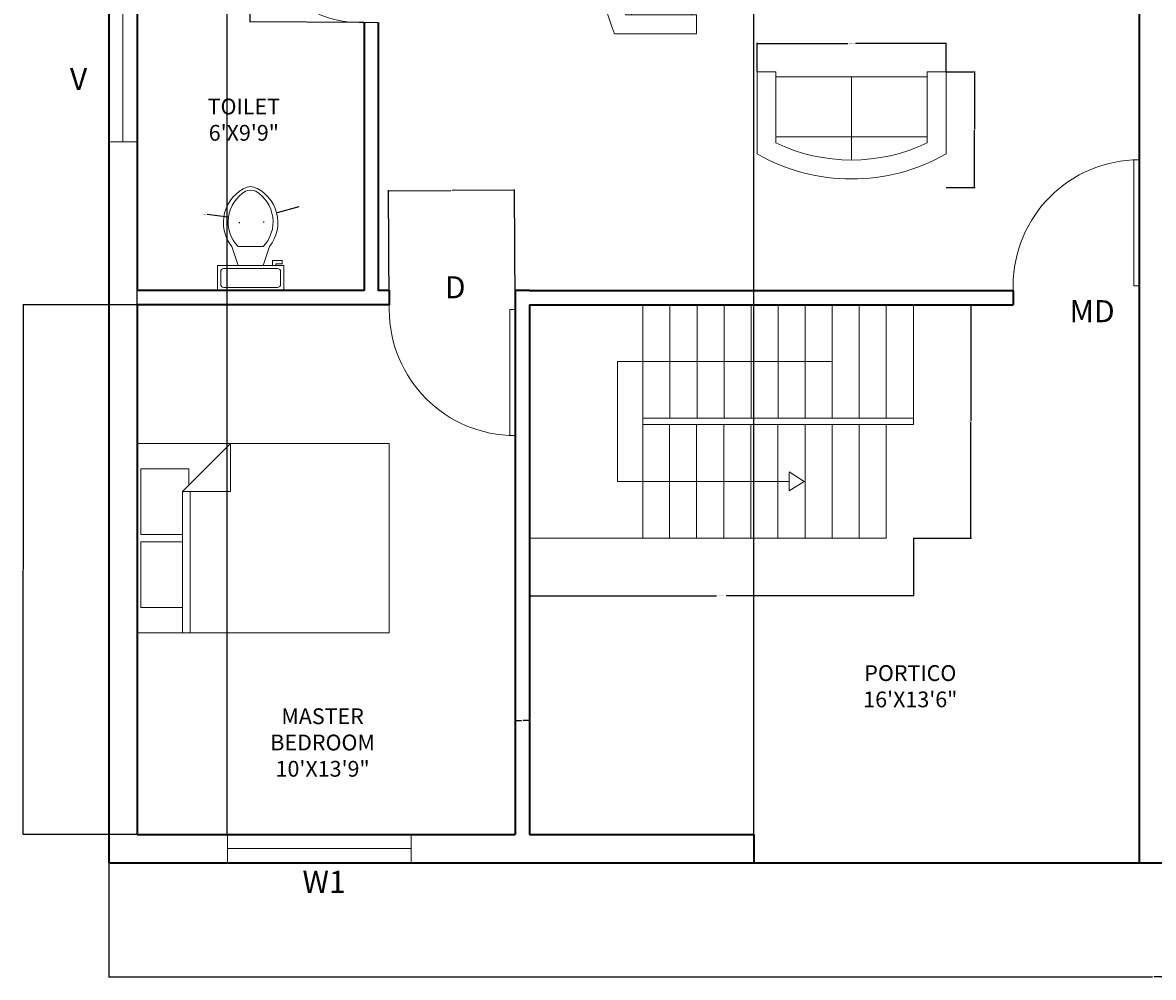
# Model space of a CAD drawing. Units: inches. Extents: x 1939 to 2674, y 558 to 1170.
# Tile 1 of 6: x 1948 to 2307, y 558 to 861. Entities that reach past the tile are written whole.
import ezdxf

# ---------------------------------------------------------------- set-up
doc = ezdxf.new("R2010")
doc.units = ezdxf.units.IN
for name, color, linetype, lineweight in [('A-ANNO-DIMS', 2, 'Continuous', 18), ('A-ANNO-TEXT', 7, 'Continuous', 18), ('A-AREA-IDEN', 7, 'Continuous', 18), ('A-DOOR', 3, 'Continuous', 18), ('A-FLOR-FIXT', 9, 'Continuous', 18), ('A-FLOR-STRS', 7, 'Continuous', 18), ('A-FURN', 8, 'Continuous', 13), ('A-GLAZ', 4, 'Continuous', 18), ('A-WALL', 7, 'Continuous', 35)]:
    doc.layers.add(name, color=color, linetype=linetype, lineweight=lineweight)
doc.styles.get("Standard").update_dxf_attribs({"font": 'arial.ttf'})
doc.dimstyles.get("Standard").update_dxf_attribs({"dimtxt": 0.18, "dimasz": 0.18, "dimexe": 0.18, "dimexo": 0.0625, "dimgap": 0.09, "dimtad": 0, "dimtih": 1, "dimtoh": 1, "dimdec": 4, "dimzin": 0, "dimdsep": 46, "dimtxsty": 'Standard', "dimcen": 0.09, "dimadec": 0, "dimazin": 0, "dimtfac": 1, "dimtdec": 4, "dimtofl": 0, "dimtmove": 0, "dimatfit": 3, "dimfxl": 1, "dimtolj": 1, "dimtzin": 0, "dimarcsym": 0})

# ---------------------------------------------------------------- blocks, each defined once
blk = doc.blocks.new('Sofa - Roundback 7 ft.')
for p, q in [((-12.00002, -32.4421), (-12.00003, -6.5971)), ((11.99997, -32.4421), (11.99998, -6.5971)), ((-36.000027, -34), (-36.000027, -11.4696)), ((-35.999844, -13.3819), (35.9998, -13.3819)), ((35.99998, -34), (35.99998, -11.4696)), ((-36.000027, -32.4421), (35.99998, -32.4421))]:
    blk.add_line(p, q)
for points in [[(-36.000027, -34), (-42.000027, -34), (-42.000027, -8)], [(41.99998, -8), (41.99998, -34), (35.99998, -34)]]:
    blk.add_lwpolyline(points)
for centre, radius, start, end in [((0, -114.25), 114.25, 68.43141, 111.5686), ((-0.00001, -127.1968), 121.1968, 72.72033, 107.2797)]:
    blk.add_arc(centre, radius, start, end)
blk = doc.blocks.new('Toilet - top')
for p, q in [((9.5, -6), (9.5, -2)), ((-10, -8.5), (-8, -8.5)), ((-10, -9.5), (-10, -8.5)), ((-7, -9.5), (-10, -9.5)), ((-8, -8.5), (-8, -8)), ((-7, -8), (-7, -9.5)), ((-4, -8), (-6, -14)), ((4, -8), (6, -14)), ((4, -14), (-4, -14))]:
    blk.add_line(p, q)
blk.add_lwpolyline([(10.5, -8), (10.5, 0), (-10.5, 0), (-10.5, -8)], close=True)
for points in [[(-9.5, -2), (-9.5, -6)], [(8.5, -1), (-8.5, -1)], [(-8.5, -7), (8.5, -7)]]:
    blk.add_lwpolyline(points)
for centre, radius, start, end in [((-8.62, -1.88), 0.884, 81.8699, 188.1301), ((8.62, -1.88), 0.884, 351.8699, 98.1301), ((-8.62, -6.12), 0.884, 171.8699, 278.1301), ((8.62, -6.12), 0.884, 261.8699, 8.1301), ((3.52, -21.58), 12.17, 141.4691, 247.9714), ((4.2, -21.82), 11.33, 136.3677, 238.9468), ((-3.52, -21.58), 12.17, 292.0284, 38.5307), ((-4.2, -21.82), 11.33, 301.053, 43.6321), ((0, -27.88), 4, 245.7318, 294.2682), ((0, -29), 4, 254.8605, 285.1395)]:
    blk.add_arc(centre, radius, start, end)
blk = doc.blocks.new('Bed - Queen')
for p, q in [((0, -80.00003), (0, 0)), ((0, 0), (59.99999, 0)), ((59.99999, 0), (59.99999, -80.00003)), ((7.99999, -1.2), (28.79998, -1.2)), ((7.99999, -14.4), (7.99999, -1.2)), ((28.79998, -1.2), (28.79998, -14.4)), ((31.19999, -1.2), (51.99999, -1.2)), ((31.19999, -14.4), (31.19999, -1.2)), ((51.99999, -1.2), (51.99999, -16.4)), ((0, -14.4), (44.8, -14.4)), ((44.8, -16.8), (0, -16.8)), ((59.99999, -29.6), (44.8, -14.4)), ((44.8, -14.4), (44.8, -29.6)), ((51.99999, -16.4), (46.79936, -16.4)), ((44.8, -29.6), (59.99999, -29.6)), ((59.99999, -80.00003), (0, -80.00003))]:
    blk.add_line(p, q)
blk = doc.blocks.new('Sofa - Roundback Loveseat 5 ft.')
for p, q in [((0, -32.44198), (0, -5.99998)), ((-24, -33.99998), (-24, -11.46958)), ((-23.9998, -13.38178), (23.99986, -13.38178)), ((24.00004, -33.99998), (24.00004, -11.46958)), ((-24, -32.44198), (24.00004, -32.44198))]:
    blk.add_line(p, q)
for points in [[(-24, -33.99998), (-30, -33.99998), (-30, -7.99998)], [(30.00004, -7.99998), (30.00004, -33.99998), (24.00004, -33.99998)]]:
    blk.add_lwpolyline(points)
for centre, radius, start, end in [((0, -60.24998), 60.24998, 60.13715, 119.8628), ((0, -61.38438), 55.38444, 64.32083, 115.6792)]:
    blk.add_arc(centre, radius, start, end)
blk = doc.blocks.new('*U12')
for p, q in [((0, 0), (0, -6)), ((-32, 0), (-32, -6))]:
    blk.add_line(p, q)
blk.add_lwpolyline([(0, 0), (0, 32), (-1.75, 32), (-1.75, 0)], close=True)
blk.add_arc((0, 0), 32, 90, 180)
blk = doc.blocks.new('*U11')
for p, q in [((0, 0), (0, -6)), ((-40, 0), (-40, -6))]:
    blk.add_line(p, q)
blk.add_lwpolyline([(0, 0), (0, 40), (-1.75, 40), (-1.75, 0)], close=True)
blk.add_arc((0, 0), 40, 90, 180)
blk = doc.blocks.new('VENT-TOILET')
for p, q in [((0, 41.35), (9, 41.35)), ((4.5, 0), (4.5, 41.35)), ((0, 0), (9, 0))]:
    blk.add_line(p, q)
blk = doc.blocks.new('WIN-MASTER')
for p, q in [((0, 9), (0, 0)), ((58.35, 9), (58.35, 0)), ((0, 4.5), (58.35, 4.5))]:
    blk.add_line(p, q)
blk = doc.blocks.new('STAIR-RETURN-PORTICO')
for p, q in [((36, 74), (36, 0)), ((44.58, 74), (44.58, 38)), ((53.17, 74), (53.17, 38)), ((61.75, 74), (61.75, 38)), ((70.33, 74), (70.33, 38)), ((78.92, 74), (78.92, 38)), ((87.5, 74), (87.5, 38)), ((96.08, 74), (96.08, 38)), ((104.66, 74), (104.66, 38)), ((113.25, 74), (113.25, 38)), ((121.83, 74), (121.83, 36)), ((96.08, 56), (27.96, 56)), ((27.96, 56), (27.96, 18)), ((36, 38), (121.83, 38)), ((36, 36), (121.83, 36)), ((44.45, 36), (44.45, 0)), ((53.05, 36), (53.05, 0)), ((61.65, 36), (61.65, 0)), ((70.25, 36), (70.25, 0)), ((78.85, 36), (78.85, 0)), ((87.45, 36), (87.45, 0)), ((96.05, 36), (96.05, 0)), ((104.65, 36), (104.65, 0)), ((113.25, 36), (113.25, 0)), ((27.96, 18), (82.39, 18)), ((82.39, 18), (82.39, 21)), ((82.39, 21), (87.13, 18)), ((82.39, 18), (82.39, 15)), ((82.39, 15), (87.13, 18)), ((0, 0), (113.25, 0))]:
    blk.add_line(p, q)
blk = doc.blocks.new('*D22')
at = {"layer": 'A-ANNO-DIMS', "color": 0, "lineweight": -2, "transparency": 16777216}
for p, q in [((2180.76, 845.08), (2180.76, 854.2)), ((2240.76, 845.08), (2240.76, 854.2)), ((2180.94, 854.02), (2209.53, 854.02)), ((2240.58, 854.02), (2211.98, 854.02))]:
    blk.add_line(p, q, dxfattribs=at)
at = {"layer": 'A-ANNO-DIMS', "color": 0, "transparency": 16777216}
for points in [[(2180.94, 854.05), (2180.94, 853.99), (2180.76, 854.02)], [(2240.58, 854.05), (2240.58, 853.99), (2240.76, 854.02)]]:
    blk.add_solid(points, dxfattribs=at)
at = {"layer": 'Defpoints', "color": 0, "transparency": 16777216}
for p in [(2240.76, 854.02), (2180.76, 845.02), (2240.76, 845.02)]:
    blk.add_point(p, dxfattribs=at)
at = {"layer": 'A-ANNO-DIMS', "color": 0, "transparency": 16777216, "insert": (2210.76, 854.02), "char_height": 0.18, "attachment_point": 5}
blk.add_mtext('\\A1;LOVESEAT 60 TYP.', dxfattribs=at)
blk = doc.blocks.new('*D23')
at = {"layer": 'A-ANNO-DIMS', "color": 0, "lineweight": -2, "transparency": 16777216}
for p, q in [((2240.82, 845.02), (2249.94, 845.02)), ((2249.76, 844.84), (2249.76, 826.86)), ((2249.76, 808.53), (2249.76, 826.5)), ((2240.82, 808.35), (2249.94, 808.35))]:
    blk.add_line(p, q, dxfattribs=at)
at = {"layer": 'A-ANNO-DIMS', "color": 0, "transparency": 16777216}
for points in [[(2249.73, 844.84), (2249.79, 844.84), (2249.76, 845.02)], [(2249.73, 808.53), (2249.79, 808.53), (2249.76, 808.35)]]:
    blk.add_solid(points, dxfattribs=at)
at = {"layer": 'Defpoints', "color": 0, "transparency": 16777216}
for p in [(2240.76, 845.02), (2240.76, 808.35), (2249.76, 808.35)]:
    blk.add_point(p, dxfattribs=at)
at = {"layer": 'A-ANNO-DIMS', "color": 0, "transparency": 16777216, "insert": (2249.76, 826.68), "char_height": 0.18, "attachment_point": 5}
blk.add_mtext('\\A1;37 TYP.', dxfattribs=at)
blk = doc.blocks.new('*D48')
at = {"layer": 'A-ANNO-DIMS', "color": 0, "lineweight": -2, "transparency": 16777216}
for p, q in [((2108.55, 697.05), (2108.55, 678.66)), ((2230.38, 697.05), (2230.38, 678.66)), ((2108.73, 678.84), (2167.91, 678.84)), ((2230.2, 678.84), (2171.02, 678.84))]:
    blk.add_line(p, q, dxfattribs=at)
at = {"layer": 'A-ANNO-DIMS', "color": 0, "transparency": 16777216}
for points in [[(2108.73, 678.87), (2108.73, 678.81), (2108.55, 678.84)], [(2230.2, 678.87), (2230.2, 678.81), (2230.38, 678.84)]]:
    blk.add_solid(points, dxfattribs=at)
at = {"layer": 'Defpoints', "color": 0, "transparency": 16777216}
for p in [(2108.55, 697.11), (2230.38, 697.11), (2230.38, 678.84)]:
    blk.add_point(p, dxfattribs=at)
at = {"layer": 'A-ANNO-DIMS', "color": 0, "transparency": 16777216, "insert": (2169.46, 678.84), "char_height": 0.18, "attachment_point": 5}
blk.add_mtext('\\A1;RETURN STAIR 122 TYP.', dxfattribs=at)
blk = doc.blocks.new('*D49')
at = {"layer": 'A-ANNO-DIMS', "color": 0, "lineweight": -2, "transparency": 16777216}
for p, q in [((2230.44, 771.11), (2248.83, 771.11)), ((2248.65, 770.93), (2248.65, 734.29)), ((2248.65, 697.29), (2248.65, 733.93)), ((2230.44, 697.11), (2248.83, 697.11))]:
    blk.add_line(p, q, dxfattribs=at)
at = {"layer": 'A-ANNO-DIMS', "color": 0, "transparency": 16777216}
for points in [[(2248.62, 770.93), (2248.68, 770.93), (2248.65, 771.11)], [(2248.62, 697.29), (2248.68, 697.29), (2248.65, 697.11)]]:
    blk.add_solid(points, dxfattribs=at)
at = {"layer": 'Defpoints', "color": 0, "transparency": 16777216}
for p in [(2230.38, 771.11), (2248.65, 771.11), (2230.38, 697.11)]:
    blk.add_point(p, dxfattribs=at)
at = {"layer": 'A-ANNO-DIMS', "color": 0, "transparency": 16777216, "insert": (2248.65, 734.11), "char_height": 0.18, "attachment_point": 5}
blk.add_mtext('\\A1;74 TYP.', dxfattribs=at)
blk = doc.blocks.new('*D51')
at = {"layer": 'A-ANNO-DIMS', "color": 0, "lineweight": -2, "transparency": 16777216}
for p, q in [((1975.05, 594.05), (1975.05, 557.78)), ((2638.05, 594.05), (2638.05, 557.78)), ((1975.23, 557.96), (2306.26, 557.96)), ((2637.87, 557.96), (2306.84, 557.96))]:
    blk.add_line(p, q, dxfattribs=at)
at = {"layer": 'A-ANNO-DIMS', "color": 0, "transparency": 16777216}
for points in [[(1975.23, 557.99), (1975.23, 557.93), (1975.05, 557.96)], [(2637.87, 557.99), (2637.87, 557.93), (2638.05, 557.96)]]:
    blk.add_solid(points, dxfattribs=at)
at = {"layer": 'Defpoints', "color": 0, "transparency": 16777216}
for p in [(1975.05, 594.11), (2638.05, 594.11), (2638.05, 557.96)]:
    blk.add_point(p, dxfattribs=at)
at = {"layer": 'A-ANNO-DIMS', "color": 0, "transparency": 16777216, "insert": (2306.55, 557.96), "char_height": 0.18, "attachment_point": 5}
blk.add_mtext('\\A1;663', dxfattribs=at)
blk = doc.blocks.new('*D53')
at = {"layer": 'A-ANNO-DIMS', "color": 0, "lineweight": -2, "transparency": 16777216}
for p, q in [((2064.05, 771.17), (2063.82, 807.44)), ((2103.64, 807.51), (2084.04, 807.39)), ((2104.05, 771.42), (2103.82, 807.69)), ((2064, 807.26), (2083.6, 807.38))]:
    blk.add_line(p, q, dxfattribs=at)
at = {"layer": 'A-ANNO-DIMS', "color": 0, "transparency": 16777216}
for points in [[(2103.64, 807.54), (2103.64, 807.48), (2103.82, 807.51)], [(2064, 807.29), (2064, 807.23), (2063.82, 807.26)]]:
    blk.add_solid(points, dxfattribs=at)
at = {"layer": 'Defpoints', "color": 0, "transparency": 16777216}
for p in [(2103.82, 807.51), (2064.05, 771.11), (2104.05, 771.36)]:
    blk.add_point(p, dxfattribs=at)
at = {"layer": 'A-ANNO-DIMS', "color": 0, "transparency": 16777216, "insert": (2083.82, 807.38), "char_height": 0.18, "attachment_point": 5}
blk.add_mtext('\\A1;40', dxfattribs=at)
blk = doc.blocks.new('*D55')
at = {"layer": 'A-ANNO-DIMS', "color": 0, "lineweight": -2, "transparency": 16777216}
for p, q in [((2056.24, 892.61), (2019.97, 892.89)), ((2020.15, 892.71), (2020.03, 877.07)), ((2019.9, 861.07), (2020.02, 876.71)), ((2055.99, 860.61), (2019.72, 860.89))]:
    blk.add_line(p, q, dxfattribs=at)
at = {"layer": 'A-ANNO-DIMS', "color": 0, "transparency": 16777216}
for points in [[(2020.12, 892.71), (2020.18, 892.71), (2020.15, 892.89)], [(2019.87, 861.07), (2019.93, 861.07), (2019.9, 860.89)]]:
    blk.add_solid(points, dxfattribs=at)
at = {"layer": 'Defpoints', "color": 0, "transparency": 16777216}
for p in [(2020.15, 892.89), (2056.3, 892.61), (2056.05, 860.61)]:
    blk.add_point(p, dxfattribs=at)
at = {"layer": 'A-ANNO-DIMS', "color": 0, "transparency": 16777216, "insert": (2020.02, 876.89), "char_height": 0.18, "attachment_point": 5}
blk.add_mtext('\\A1;32', dxfattribs=at)
blk = doc.blocks.new('*D58')
at = {"layer": 'A-ANNO-DIMS', "color": 0, "lineweight": -2, "transparency": 16777216}
for p, q in [((2179.79, 603.17), (2179.79, 1170.44)), ((2179.97, 1170.26), (2240.46, 1170.26)), ((2301.87, 1170.26), (2241.37, 1170.26)), ((2302.05, 594.17), (2302.05, 1170.44))]:
    blk.add_line(p, q, dxfattribs=at)
at = {"layer": 'A-ANNO-DIMS', "color": 0, "transparency": 16777216}
for points in [[(2179.97, 1170.29), (2179.97, 1170.23), (2179.79, 1170.26)], [(2301.87, 1170.29), (2301.87, 1170.23), (2302.05, 1170.26)]]:
    blk.add_solid(points, dxfattribs=at)
at = {"layer": 'Defpoints', "color": 0, "transparency": 16777216}
for p in [(2302.05, 1170.26), (2179.79, 603.11), (2302.05, 594.11)]:
    blk.add_point(p, dxfattribs=at)
at = {"layer": 'A-ANNO-DIMS', "color": 0, "transparency": 16777216, "insert": (2240.92, 1170.26), "char_height": 0.18, "attachment_point": 5}
blk.add_mtext('\\A1;122.26', dxfattribs=at)
blk = doc.blocks.new('*D61')
at = {"layer": 'A-ANNO-DIMS', "color": 0, "lineweight": -2, "transparency": 16777216}
for p, q in [((1984.05, 603.17), (1984.05, 1170.44)), ((1984.23, 1170.26), (1997.89, 1170.26)), ((2012.48, 1170.26), (1998.82, 1170.26)), ((2012.66, 603.17), (2012.66, 1170.44))]:
    blk.add_line(p, q, dxfattribs=at)
at = {"layer": 'A-ANNO-DIMS', "color": 0, "transparency": 16777216}
for points in [[(1984.23, 1170.29), (1984.23, 1170.23), (1984.05, 1170.26)], [(2012.48, 1170.29), (2012.48, 1170.23), (2012.66, 1170.26)]]:
    blk.add_solid(points, dxfattribs=at)
at = {"layer": 'Defpoints', "color": 0, "transparency": 16777216}
for p in [(2012.66, 1170.26), (1984.05, 603.11), (2012.66, 603.11)]:
    blk.add_point(p, dxfattribs=at)
at = {"layer": 'A-ANNO-DIMS', "color": 0, "transparency": 16777216, "insert": (1998.36, 1170.26), "char_height": 0.18, "attachment_point": 5}
blk.add_mtext('\\A1;28.616', dxfattribs=at)
blk = doc.blocks.new('*D66')
at = {"layer": 'A-ANNO-DIMS', "color": 0, "lineweight": -2, "transparency": 16777216}
for p, q in [((1983.99, 771.11), (1947.72, 771.11)), ((1947.9, 770.93), (1947.9, 687.29)), ((1947.9, 603.29), (1947.9, 686.93)), ((1983.99, 603.11), (1947.72, 603.11))]:
    blk.add_line(p, q, dxfattribs=at)
at = {"layer": 'A-ANNO-DIMS', "color": 0, "transparency": 16777216}
for points in [[(1947.87, 770.93), (1947.93, 770.93), (1947.9, 771.11)], [(1947.87, 603.29), (1947.93, 603.29), (1947.9, 603.11)]]:
    blk.add_solid(points, dxfattribs=at)
at = {"layer": 'Defpoints', "color": 0, "transparency": 16777216}
for p in [(1947.9, 771.11), (1984.05, 771.11), (1984.05, 603.11)]:
    blk.add_point(p, dxfattribs=at)
at = {"layer": 'A-ANNO-DIMS', "color": 0, "transparency": 16777216, "insert": (1947.9, 687.11), "char_height": 0.18, "attachment_point": 5}
blk.add_mtext('\\A1;168', dxfattribs=at)
blk = doc.blocks.new('*D69')
at = {"layer": 'A-ANNO-DIMS', "color": 0, "lineweight": -2, "transparency": 16777216}
for p, q in [((2104.05, 603.17), (2104.05, 639.44)), ((2104.23, 639.26), (2106.04, 639.26)), ((2108.37, 639.26), (2106.56, 639.26)), ((2108.55, 603.17), (2108.55, 639.44))]:
    blk.add_line(p, q, dxfattribs=at)
at = {"layer": 'A-ANNO-DIMS', "color": 0, "transparency": 16777216}
for points in [[(2104.23, 639.29), (2104.23, 639.23), (2104.05, 639.26)], [(2108.37, 639.29), (2108.37, 639.23), (2108.55, 639.26)]]:
    blk.add_solid(points, dxfattribs=at)
at = {"layer": 'Defpoints', "color": 0, "transparency": 16777216}
for p in [(2108.55, 639.26), (2104.05, 603.11), (2108.55, 603.11)]:
    blk.add_point(p, dxfattribs=at)
at = {"layer": 'A-ANNO-DIMS', "color": 0, "transparency": 16777216, "insert": (2106.3, 639.26), "char_height": 0.18, "attachment_point": 5}
blk.add_mtext('\\A1;4.5', dxfattribs=at)
blk = doc.blocks.new('*D77')
at = {"layer": 'A-ANNO-DIMS', "color": 0, "lineweight": -2, "transparency": 16777216}
for p, q in [((2035.36, 802.14), (2028.47, 800.33)), ((2016.44, 797.19), (2016.62, 797.19)), ((2016.53, 797.1), (2016.53, 797.28))]:
    blk.add_line(p, q, dxfattribs=at)
at = {"layer": 'A-ANNO-DIMS', "color": 0, "transparency": 16777216}
blk.add_solid([(2028.46, 800.36), (2028.48, 800.3), (2028.3, 800.28)], dxfattribs=at)
at = {"layer": 'Defpoints', "color": 0, "transparency": 16777216}
for p in [(2028.3, 800.28), (2016.53, 797.19)]:
    blk.add_point(p, dxfattribs=at)
at = {"layer": 'A-ANNO-DIMS', "color": 0, "transparency": 16777216, "insert": (2036.04, 802.14), "char_height": 0.18, "attachment_point": 5}
blk.add_mtext('\\A1;4X R12.17', dxfattribs=at)
blk = doc.blocks.new('*D78')
at = {"layer": 'A-ANNO-DIMS', "color": 0, "lineweight": -2, "transparency": 16777216}
for p, q in [((2006.28, 799.84), (2012.84, 798.96)), ((2024.16, 797.43), (2024.34, 797.43)), ((2024.25, 797.34), (2024.25, 797.52))]:
    blk.add_line(p, q, dxfattribs=at)
at = {"layer": 'A-ANNO-DIMS', "color": 0, "transparency": 16777216}
blk.add_solid([(2012.85, 798.99), (2012.84, 798.93), (2013.02, 798.94)], dxfattribs=at)
at = {"layer": 'Defpoints', "color": 0, "transparency": 16777216}
for p in [(2013.02, 798.94), (2024.25, 797.43)]:
    blk.add_point(p, dxfattribs=at)
at = {"layer": 'A-ANNO-DIMS', "color": 0, "transparency": 16777216, "insert": (2005.61, 799.84), "char_height": 0.18, "attachment_point": 5}
blk.add_mtext('\\A1;4X R11.33', dxfattribs=at)

msp = doc.modelspace()

# ---------------------------------------------------------------- linework, layer by layer
at = {"layer": 'A-WALL'}
for p, q in [((1975.0479, 1134.1102), (1975.0479, 594.1102)), ((2302.048, 1017.1102), (2302.048, 771.1102)), ((1984.0479, 892.6102), (1984.0479, 775.6102)), ((2056.048, 860.6102), (2056.048, 775.6102)), ((2060.548, 860.6102), (2060.548, 775.6102)), ((2056.048, 775.6102), (1984.0479, 775.6102)), ((2064.048, 775.6102), (2060.548, 775.6102)), ((2064.048, 775.6102), (2064.048, 771.1102)), ((2104.048, 775.6102), (2104.048, 603.1102)), ((2108.548, 775.6102), (2104.048, 775.6102)), ((2108.548, 775.6102), (2262.048, 775.6102)), ((2262.048, 775.6102), (2262.048, 771.1102)), ((2262.048, 775.6102), (2262.048, 771.1102)), ((2064.048, 771.1102), (1984.0479, 771.1102)), ((1984.0479, 771.1102), (1984.0479, 603.1102)), ((2108.548, 771.1102), (2108.548, 603.1102)), ((2108.548, 771.1102), (2262.048, 771.1102)), ((2302.048, 771.1102), (2302.048, 594.1102)), ((1984.0479, 603.1102), (2104.048, 603.1102)), ((2108.548, 603.1102), (2179.7888, 603.1102)), ((2179.7888, 603.1102), (2179.7888, 594.1102)), ((1975.0479, 594.1102), (2638.048, 594.1102))]:
    msp.add_line(p, q, dxfattribs=at)

# ---------------------------------------------------------------- block references
at = {"layer": 'A-DOOR', "rotation": 90}
msp.add_blockref('*U12', (2054.548, 892.6102), dxfattribs=at)
at = {"layer": 'A-DOOR'}
msp.add_blockref('*U11', (2302.048, 777.1102), dxfattribs=at)
at = {"layer": 'A-DOOR', "xscale": -1, "rotation": 180}
msp.add_blockref('*U11', (2104.048, 769.6102), dxfattribs=at)
at = {"layer": 'A-FLOR-FIXT', "rotation": 180}
msp.add_blockref('Toilet - top', (2020.048, 775.6102), dxfattribs=at)
at = {"layer": 'A-FLOR-STRS'}
msp.add_blockref('STAIR-RETURN-PORTICO', (2108.548, 697.1102), dxfattribs=at)
at = {"layer": 'A-FURN', "rotation": 90}
for name, p in [('Sofa - Roundback 7 ft.', (2127.5709, 899.043)), ('Bed - Queen', (1984.0479, 667.1037))]:
    msp.add_blockref(name, p, dxfattribs=at)
at = {"layer": 'A-FURN', "xscale": -1, "rotation": 180}
msp.add_blockref('Sofa - Roundback Loveseat 5 ft.', (2210.7572, 811.0152), dxfattribs=at)
at = {"layer": 'A-GLAZ'}
for name, p in [('VENT-TOILET', (1975.0479, 822.7612)), ('WIN-MASTER', (2012.6641, 594.1102))]:
    msp.add_blockref(name, p, dxfattribs=at)

# ---------------------------------------------------------------- texts
at = {"layer": 'A-ANNO-TEXT', "char_height": 7, "attachment_point": 1}
for s, insert in [('\\pxqc;V', (1954.5035, 846.2453)), ('\\pxqc;D', (2074.031, 780.1743)), ('\\pxqc;MD', (2276.1621, 772.5911)), ('\\pxqc;W1', (2032.4101, 591.5736))]:
    msp.add_mtext_dynamic_manual_height_columns(s, width=21.893501, gutter_width=12.5, heights=[0], dxfattribs=dict(at, insert=insert))
at = {"layer": 'A-AREA-IDEN', "char_height": 5, "attachment_point": 1}
for s, insert in [('\\pxqc;TOILET\\P6\'X9\'9"', (1998.3374, 836.4962)), ('\\pxqc;PORTICO\\P16\'X13\'6"', (2209.8478, 656.7886)), ('\\pxqc;MASTER\\PBEDROOM\\P10\'X13\'9"', (2023.3387, 643.1082))]:
    msp.add_mtext_dynamic_manual_height_columns(s, width=39.116177, gutter_width=12.5, heights=[0], dxfattribs=dict(at, insert=insert))

# ---------------------------------------------------------------- dimensions: what is measured, and where the dimension line sits
at = {"layer": 'A-ANNO-DIMS'}
for base, p1, p2, override, picture, middle in [((2012.6641, 1170.2602), (1984.0479, 603.1102), (2012.6641, 603.1102), {"dimdec": 3, "dimlfac": 1, "dimrnd": 0, "dimzin": 0, "dimdsep": 46, "dimlunit": 2}, '*D61', (1998.356, 1170.2602)), ((2302.048, 1170.2602), (2179.7888, 603.1102), (2302.048, 594.1102), {"dimdec": 2, "dimlfac": 1, "dimrnd": 0, "dimzin": 0, "dimdsep": 46, "dimlunit": 2}, '*D58', (2240.9184, 1170.2602)), ((2108.548, 639.2602), (2104.048, 603.1102), (2108.548, 603.1102), {"dimdec": 1, "dimlfac": 1, "dimrnd": 0, "dimzin": 0, "dimdsep": 46, "dimlunit": 2}, '*D69', (2106.298, 639.2602)), ((2638.048, 557.9602), (1975.0479, 594.1102), (2638.048, 594.1102), {"dimdec": 0, "dimlfac": 1, "dimrnd": 0, "dimzin": 0, "dimdsep": 46, "dimlunit": 2}, '*D51', (2306.548, 557.9602))]:
    dim = msp.add_linear_dim(base=base, p1=p1, p2=p2, dimstyle='Standard', override=override, dxfattribs=at)
    dim.commit()
    dim.dimension.update_dxf_attribs({"geometry": picture, "text_midpoint": middle})
for base, p1, p2, angle, picture, middle in [((2020.1491, 892.8926), (2056.048, 860.6102), (2056.298, 892.6102), 89.552386, '*D55', (2020.0241, 876.8926)), ((2103.822, 807.5095), (2064.048, 771.1102), (2104.048, 771.3602), 0.358094, '*D53', (2083.822, 807.3845)), ((1947.898, 771.1102), (1984.0479, 603.1102), (1984.0479, 771.1102), 90, '*D66', (1947.898, 687.1102))]:
    dim = msp.add_linear_dim(base=base, p1=p1, p2=p2, angle=angle, dimstyle='Standard', override={"dimdec": 0, "dimlfac": 1, "dimrnd": 0, "dimzin": 0, "dimdsep": 46, "dimlunit": 2}, dxfattribs=at)
    dim.commit()
    dim.dimension.update_dxf_attribs({"geometry": picture, "text_midpoint": middle})
for base, p1, p2, text, picture, middle in [((2240.7573, 854.0152), (2180.7572, 845.0152), (2240.7573, 845.0152), 'LOVESEAT <> TYP.', '*D22', (2210.7573, 854.0152)), ((2230.3788, 678.8356), (2108.548, 697.1102), (2230.3788, 697.1102), 'RETURN STAIR <> TYP.', '*D48', (2169.4634, 678.8356))]:
    dim = msp.add_linear_dim(base=base, p1=p1, p2=p2, text=text, dimstyle='Standard', override={"dimdec": 0, "dimlfac": 1, "dimrnd": 0, "dimzin": 0, "dimdsep": 46, "dimlunit": 2}, dxfattribs=at)
    dim.commit()
    dim.dimension.update_dxf_attribs({"geometry": picture, "text_midpoint": middle})
for base, p1, p2, angle, picture, middle in [((2249.7573, 808.3486), (2240.7573, 845.0152), (2240.7573, 808.3486), 270, '*D23', (2249.7573, 826.6819)), ((2248.6534, 771.1102), (2230.3788, 697.1102), (2230.3788, 771.1102), 90, '*D49', (2248.6534, 734.1102))]:
    dim = msp.add_linear_dim(base=base, p1=p1, p2=p2, angle=angle, text='<> TYP.', dimstyle='Standard', override={"dimdec": 0, "dimlfac": 1, "dimrnd": 0, "dimzin": 0, "dimdsep": 46, "dimlunit": 2}, dxfattribs=at)
    dim.commit()
    dim.dimension.update_dxf_attribs({"geometry": picture, "text_midpoint": middle})
for center, mpoint, picture, middle in [((2016.5284, 797.1907), (2028.298, 800.283), '*D77', (2035.3597, 802.1384)), ((2024.2478, 797.4276), (2013.0197, 798.937), '*D78', (2006.2828, 799.8427))]:
    dim = msp.add_radius_dim(center=center, mpoint=mpoint, text='4X <>', dimstyle='Standard', override={"dimdec": 2, "dimlfac": 1, "dimrnd": 0, "dimzin": 0, "dimdsep": 46, "dimlunit": 2}, dxfattribs=at)
    dim.commit()
    dim.dimension.update_dxf_attribs({"geometry": picture, "text_midpoint": middle, "dimtype": 164})

doc.saveas('drawing.dxf')
